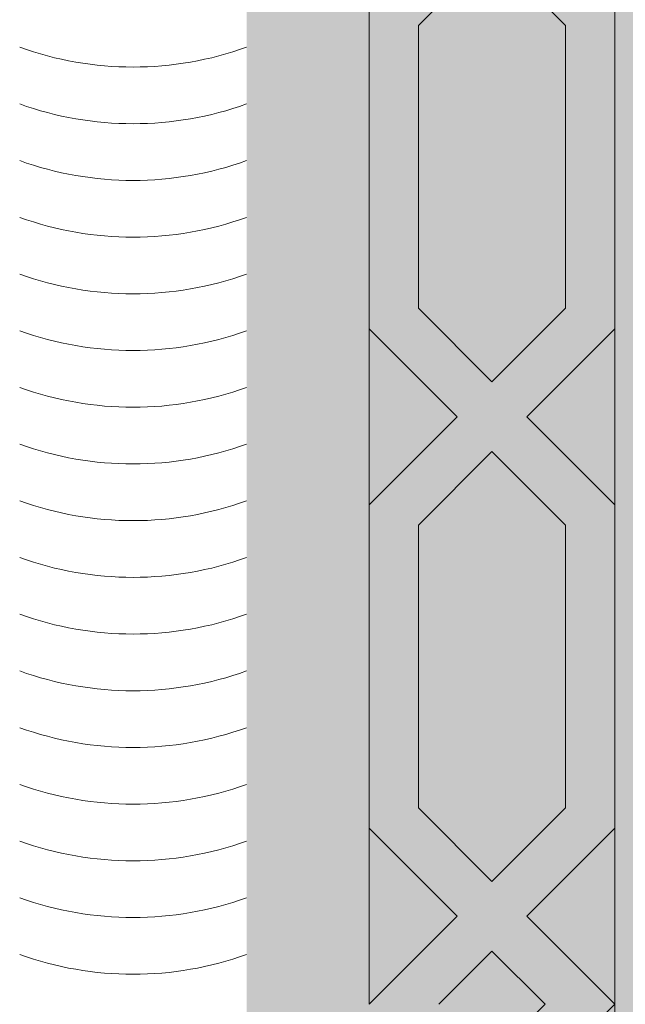
# Model space of a CAD drawing. Units: inches. Extents: x 844 to 2234, y 346 to 1084.
# Tile 56 of 93: x 1861.148 to 1864.294, y 701.365 to 706.48. Entities that reach past the tile are written whole.
import ezdxf

# ---------------------------------------------------------------- set-up
doc = ezdxf.new("R2010")
doc.units = ezdxf.units.IN
doc.header["$MEASUREMENT"] = 0
doc.layers.add('furniture', color=8, linetype='Continuous', lineweight=18)
doc.layers.add('RA-AP-01$0$INT', color=35, linetype='Continuous', lineweight=5)
doc.layers.add('RA-AP-01$0$FURN', color=3, linetype='Continuous')

# ---------------------------------------------------------------- blocks, each defined once
blk = doc.blocks.new('A$C18D01794')
at = {"layer": 'RA-AP-01$0$INT'}
h = blk.add_hatch(color=256, dxfattribs=at)
h.paths.add_polyline_path([(4.355206456958071, -6.156712009588037), (4.355206456958071, -8.056712009588038), (5.455206456958072, -8.056712009588038), (5.455206456958072, -6.156712009588037)])
h.paths.add_polyline_path([(4.405206456958072, -8.006712009588039), (4.405206456958072, -6.206712009588038), (5.405206456958072, -6.206712009588038), (5.405206456958072, -8.006712009588039)], flags=16)
h = blk.add_hatch(color=256, dxfattribs=at)
h.paths.add_polyline_path([(4.469348592586677, -7.07085414521094), (4.505206456958073, -7.03499628085108), (4.505206456958071, -7.106712009593861)])
h.paths.add_polyline_path([(4.455206456960671, -7.084996280832395), (4.476922185709333, -7.106712009588038), (4.433490728198045, -7.106712009588038)])
h.paths.add_polyline_path([(4.405206456958073, -7.034996280813718), (4.441064321339218, -7.070854145206393), (4.40520645695807, -7.106712009576003)])
h.paths.add_polyline_path([(4.425206456989053, -6.911460746921742), (4.455206456990736, -6.881460746929706), (4.485206456989055, -6.911460746937677), (4.48520645696979, -7.026712009590022), (4.455206456965227, -7.056712009584936), (4.425206456969784, -7.026712009579853)])
h.paths.add_polyline_path([(4.505206456958073, -6.831460746955388), (4.505206456958071, -6.903176475661116), (4.469348592616738, -6.867318611308251)])
h.paths.add_polyline_path([(4.425206456964688, -6.707925213036777), (4.455206456964794, -6.677925213027025), (4.485206456964689, -6.707925213017265), (4.485206456983951, -6.823176475683938), (4.455206456990736, -6.853176475686799), (4.425206456983956, -6.823176475689667)])
h.paths.add_polyline_path([(4.425206456974126, -6.504389679118949), (4.455206456959092, -6.474389679124341), (4.485206456974132, -6.504389679129721), (4.485206456993396, -6.619640941768059), (4.45520645699153, -6.649640941779566), (4.425206456993394, -6.619640941791077)])
h.paths.add_polyline_path([(4.46934859260189, -6.663783077416661), (4.505206456958071, -6.627925213048953), (4.505206456958073, -6.699640941761311)])
h.paths.add_polyline_path([(4.405206456958073, -6.627925213005104), (4.441064321354427, -6.663783077389926), (4.405206456958072, -6.699640941797813)])
h.paths.add_polyline_path([(4.405206456958072, -6.424389679139403), (4.441064321333084, -6.460247543502882), (4.405206456958072, -6.496105407889427)])
h.paths.add_polyline_path([(4.469348592580547, -6.460247543498336), (4.505206456958071, -6.424389679109282), (4.505206456958071, -6.496105407864332)])
h.paths.add_polyline_path([(4.425206456957888, -6.300854145208262), (4.45520645695415, -6.270854145221655), (4.485206456959507, -6.300854145217359), (4.48520645695824, -6.416105407863534), (4.455206456954537, -6.44610540787688), (4.425206456957888, -6.416105407889874)])
h.paths.add_polyline_path([(4.425206456957888, -6.226712009591025), (4.471064321332215, -6.226712009591025), (4.425206456957888, -6.272569873980103)])
h.paths.add_polyline_path([(4.499348592575121, -6.226712009591029), (4.636064321343707, -6.226712009591025), (4.666064321342317, -6.256712009589254), (4.636064321340932, -6.286712009591028), (4.499348592588945, -6.286712009591028), (4.469348592591685, -6.256712009584116)])
h.paths.add_polyline_path([(4.680206456964641, -6.270854145214393), (4.716064321337824, -6.306712009588038), (4.644348592591454, -6.306712009588038)])
h.paths.add_polyline_path([(4.644348592588108, -6.206712009588038), (4.716064321341167, -6.206712009588038), (4.680206456964637, -6.242569873964111)])
h.paths.add_polyline_path([(4.724348592586768, -6.226712009589824), (4.861064321340514, -6.226712009589824), (4.891064321340324, -6.256712009589255), (4.861064321340141, -6.286712009589827), (4.724348592587134, -6.286712009589821), (4.694348592586957, -6.256712009589254)])
h.paths.add_polyline_path([(4.905206456964143, -6.270854145212892), (4.941064321338827, -6.306712009588038), (4.869348592589457, -6.306712009588039)])
h.paths.add_polyline_path([(4.869348592586113, -6.206712009588038), (4.941064321342172, -6.206712009588038), (4.905206456964145, -6.242569873965612)])
h.paths.add_polyline_path([(4.949348592587774, -6.226712009589824), (5.086064321341521, -6.226712009589824), (5.116064321341329, -6.256712009589252), (5.08606432134115, -6.286712009589823), (4.949348592588145, -6.286712009589827), (4.919348592587961, -6.256712009589255)])
h.paths.add_polyline_path([(5.130206456963645, -6.270854145214393), (5.166064321336834, -6.306712009588038), (5.094348592590464, -6.306712009588038)])
h.paths.add_polyline_path([(5.094348592587119, -6.206712009588038), (5.166064321340178, -6.206712009588038), (5.130206456963651, -6.242569873964107)])
h.paths.add_polyline_path([(5.174348592584578, -6.226712009591027), (5.311064321353163, -6.226712009591027), (5.341064321336602, -6.256712009584116), (5.31106432133934, -6.286712009591028), (5.174348592587352, -6.286712009591028), (5.144348592585969, -6.256712009589254)])
h.paths.add_polyline_path([(5.325206456968778, -6.300854145217359), (5.355206456974136, -6.270854145221653), (5.385206456970396, -6.300854145208262), (5.385206456970396, -6.416105407889878), (5.355206456973747, -6.44610540787688), (5.325206456970044, -6.416105407863533)])
h.paths.add_polyline_path([(5.339348592596073, -6.226712009591029), (5.385206456970396, -6.226712009591025), (5.385206456970398, -6.272569873980105)])
h.paths.add_polyline_path([(5.325206456954155, -6.504389679129722), (5.355206456969194, -6.474389679124342), (5.38520645695416, -6.504389679118949), (5.385206456934896, -6.619640941791077), (5.355206456936758, -6.649640941779564), (5.325206456934888, -6.619640941768057)])
h.paths.add_polyline_path([(5.305206456958072, -6.424389679097139), (5.341064321347739, -6.460247543498338), (5.305206456958072, -6.496105407876472)])
h.paths.add_polyline_path([(5.369348592595204, -6.460247543502882), (5.40520645695807, -6.42438967915155), (5.405206456958072, -6.496105407877278)])
h.paths.add_polyline_path([(5.405206456958072, -6.627925213017245), (5.405206456958072, -6.69964094178567), (5.369348592573857, -6.663783077389926)])
h.paths.add_polyline_path([(5.305206456958072, -6.62792521303681), (5.341064321326393, -6.663783077416663), (5.305206456958072, -6.69964094177345)])
h.paths.add_polyline_path([(5.325206456963599, -6.707925213017267), (5.355206456963494, -6.677925213027021), (5.385206456963598, -6.707925213036775), (5.385206456944334, -6.823176475689665), (5.355206456937552, -6.853176475686797), (5.325206456944333, -6.823176475683936)])
h.paths.add_polyline_path([(5.305206456958072, -6.831460746943246), (5.341064321311551, -6.867318611308252), (5.305206456958072, -6.903176475673257)])
h.paths.add_polyline_path([(5.325206456939231, -6.911460746937672), (5.355206456937552, -6.881460746929707), (5.385206456939235, -6.911460746921742), (5.385206456958502, -7.026712009579853), (5.355206456963061, -7.056712009584934), (5.3252064569585, -7.026712009590026)])
h.paths.add_polyline_path([(5.404581768715993, -6.832085435167151, 0.001217816984214), (5.405206456958072, -6.832312009593747), (5.405206456958072, -6.90317647569123), (5.369348592563558, -6.867318611308251)])
h.paths.add_polyline_path([(5.36934859258907, -7.070854145206393), (5.40520645695807, -7.034996280825861), (5.405206456958072, -7.106712009563858)])
h.paths.add_polyline_path([(5.355206456967613, -7.084996280832394), (5.376922185730239, -7.106712009588038), (5.333490728218953, -7.106712009588036)])
h.paths.add_polyline_path([(5.30520645695807, -7.034996280838937), (5.341064321341609, -7.070854145210942), (5.305206456958074, -7.106712009606006)])
h = blk.add_hatch(color=256, dxfattribs=at)
h.paths.add_polyline_path([(4.505206456958071, -6.627925213048953), (4.46934859260189, -6.663783077416663), (4.505206456958071, -6.699640941761309), (4.505206456958071, -6.831460746955389), (4.469348592616735, -6.867318611308252), (4.505206456958071, -6.903176475661112), (4.505206456958071, -7.03499628085108), (4.469348592586679, -7.070854145210939), (4.505206456952245, -7.106712009588038), (4.476922185709333, -7.106712009588038), (4.455206456960671, -7.084996280832395), (4.433490728198047, -7.106712009588038), (4.405206456946033, -7.10671200958804), (4.441064321339216, -7.070854145206393), (4.40520645695807, -7.034996280813718), (4.405206456958072, -6.903176475703379), (4.441064321364728, -6.867318611308251), (4.40520645695807, -6.83146074691313), (4.40520645695807, -6.699640941797813), (4.441064321354429, -6.663783077389924), (4.405206456958072, -6.627925213005102), (4.405206456958072, -6.496105407889425), (4.441064321333084, -6.460247543502882), (4.405206456958072, -6.424389679139403), (4.405206456958072, -6.206712009588038), (4.644348592588106, -6.206712009588038), (4.680206456964639, -6.242569873964107), (4.716064321341165, -6.206712009588038), (4.869348592586113, -6.206712009588038), (4.905206456964143, -6.24256987396561), (4.941064321342174, -6.206712009588038), (5.094348592587118, -6.206712009588038), (5.130206456963649, -6.242569873964107), (5.166064321340178, -6.206712009588038), (5.405206456958072, -6.206712009588038), (5.405206456958072, -6.42438967915155), (5.369348592595202, -6.46024754350288), (5.40520645695807, -6.49610540787728), (5.40520645695807, -6.627925213017247), (5.369348592573859, -6.663783077389926), (5.40520645695807, -6.699640941785666), (5.40520645695807, -6.831460746925273), (5.36934859256356, -6.867318611308252), (5.405206456958072, -6.90317647569123), (5.405206456958072, -7.034996280825859), (5.369348592589068, -7.070854145206395), (5.405206456982249, -7.106712009588038), (5.376922185730244, -7.106712009588038), (5.355206456967613, -7.084996280832397), (5.333490728218955, -7.106712009588036), (5.305206456976043, -7.106712009588035), (5.341064321341609, -7.07085414521094), (5.305206456958072, -7.034996280838935), (5.305206456958072, -6.90317647567326), (5.34106432131155, -6.867318611308252), (5.305206456958072, -6.831460746943244), (5.30520645695807, -6.699640941773452), (5.341064321326395, -6.663783077416663), (5.305206456958072, -6.627925213036814), (5.305206456958072, -6.496105407876472), (5.341064321347738, -6.46024754349834), (5.305206456958072, -6.424389679097137), (5.30520645695807, -6.306712009588038), (5.166064321336834, -6.306712009588038), (5.130206456963647, -6.270854145214393), (5.094348592590464, -6.306712009588038), (4.941064321338827, -6.306712009588036), (4.905206456964145, -6.270854145212892), (4.869348592589459, -6.306712009588038), (4.716064321337822, -6.306712009588036), (4.680206456964641, -6.270854145214393), (4.644348592591453, -6.306712009588038), (4.505206456958071, -6.306712009588038), (4.505206456958071, -6.424389679109282), (4.469348592580545, -6.460247543498338), (4.505206456958071, -6.496105407864328)])
h.paths.add_polyline_path([(4.485206456974132, -6.504389679129722), (4.45520645695909, -6.474389679124341), (4.425206456974128, -6.504389679118945), (4.425206456993394, -6.619640941791079), (4.45520645699153, -6.649640941779566), (4.485206456993396, -6.619640941768059)], flags=16)
h.paths.add_polyline_path([(4.455206456954537, -6.44610540787688), (4.485206456958242, -6.416105407863534), (4.48520645695951, -6.30085414521736), (4.45520645695415, -6.270854145221653), (4.425206456957888, -6.300854145208264), (4.425206456957888, -6.41610540788988)], flags=16)
h.paths.add_polyline_path([(4.455206456964794, -6.677925213027025), (4.42520645696469, -6.707925213036777), (4.425206456983954, -6.82317647568967), (4.455206456990734, -6.853176475686797), (4.485206456983953, -6.823176475683936), (4.485206456964687, -6.707925213017265)], flags=16)
h.paths.add_polyline_path([(4.499348592588947, -6.286712009591028), (4.636064321340932, -6.286712009591028), (4.666064321342317, -6.256712009589254), (4.636064321343707, -6.226712009591027), (4.499348592575121, -6.226712009591029), (4.469348592591685, -6.256712009584118)], flags=16)
h.paths.add_polyline_path([(4.425206456957888, -6.272569873980103), (4.471064321332215, -6.226712009591025), (4.425206456957888, -6.226712009591025)], flags=16)
h.paths.add_polyline_path([(4.455206456990734, -6.881460746929709), (4.425206456989053, -6.91146074692174), (4.425206456969784, -7.026712009579853), (4.455206456965226, -7.056712009584932), (4.485206456969787, -7.026712009590026), (4.485206456989053, -6.911460746937672)], flags=16)
h.paths.add_polyline_path([(4.72434859258714, -6.286712009589821), (4.861064321340141, -6.286712009589829), (4.891064321340324, -6.256712009589254), (4.861064321340513, -6.226712009589823), (4.724348592586768, -6.226712009589823), (4.694348592586956, -6.256712009589254)], flags=16)
h.paths.add_polyline_path([(4.919348592587961, -6.256712009589254), (4.949348592588145, -6.286712009589827), (5.08606432134115, -6.286712009589823), (5.116064321341327, -6.256712009589254), (5.086064321341519, -6.226712009589824), (4.949348592587774, -6.226712009589824)], flags=16)
h.paths.add_polyline_path([(5.144348592585967, -6.256712009589254), (5.174348592587358, -6.286712009591028), (5.311064321339338, -6.286712009591028), (5.3410643213366, -6.256712009584118), (5.311064321353163, -6.226712009591029), (5.174348592584576, -6.226712009591027)], flags=16)
h.paths.add_polyline_path([(5.32520645693489, -6.619640941768055), (5.355206456936755, -6.649640941779566), (5.385206456934894, -6.619640941791079), (5.38520645695416, -6.504389679118949), (5.355206456969194, -6.474389679124341), (5.325206456954153, -6.504389679129724)], flags=16)
h.paths.add_polyline_path([(5.325206456970042, -6.416105407863534), (5.355206456973747, -6.44610540787688), (5.385206456970398, -6.416105407889876), (5.385206456970398, -6.30085414520826), (5.355206456974136, -6.270854145221653), (5.325206456968778, -6.30085414521736)], flags=16)
h.paths.add_polyline_path([(5.325206456963599, -6.707925213017265), (5.325206456944333, -6.823176475683936), (5.355206456937552, -6.853176475686797), (5.385206456944332, -6.823176475689667), (5.385206456963596, -6.707925213036773), (5.355206456963492, -6.677925213027027)], flags=16)
h.paths.add_polyline_path([(5.32520645693923, -6.911460746937674), (5.3252064569585, -7.026712009590026), (5.355206456963062, -7.056712009584934), (5.3852064569585, -7.026712009579853), (5.385206456939234, -6.911460746921738), (5.355206456937552, -6.881460746929707)], flags=16)
h.paths.add_polyline_path([(5.339348592596071, -6.226712009591029), (5.385206456970398, -6.272569873980103), (5.385206456970396, -6.226712009591027)], flags=16)
for points in [[(4.505206456958071, -6.306712009588038), (5.305206456958072, -6.306712009588038), (5.305206456958072, -7.106712009588038), (5.255206456951893, -7.10671200958804), (5.25520645694868, -6.356712009605972), (4.555206456959269, -6.356712009587461), (4.555206456956052, -7.106712009588038), (4.505206456958073, -7.106712009588038)], [(4.505206456958071, -7.906712009588039), (5.305206456958072, -7.906712009588039), (5.305206456958072, -7.106712009588038), (5.255206456951893, -7.106712009588036), (5.25520645694868, -7.856712009570104), (4.555206456959269, -7.856712009588616), (4.555206456956052, -7.106712009588038), (4.505206456958073, -7.106712009588038)], [(4.405206456958072, -7.381963272262946), (4.441064321364729, -7.346105407867824), (4.405206456958072, -7.310247543472702)]]:
    blk.add_hatch(color=256, dxfattribs=at).paths.add_polyline_path(points)
h = blk.add_hatch(color=256, dxfattribs=at)
h.paths.add_polyline_path([(4.505206456958071, -7.585498806127123), (4.46934859260189, -7.549640941759413), (4.505206456958071, -7.513783077414768), (4.505206456958071, -7.381963272220687), (4.469348592616735, -7.346105407867824), (4.505206456958071, -7.310247543514964), (4.505206456958071, -7.178427738324996), (4.469348592586679, -7.142569873965138), (4.505206456952245, -7.106712009588038), (4.476922185709333, -7.106712009588038), (4.455206456960671, -7.128427738343681), (4.433490728198047, -7.106712009588038), (4.405206456946033, -7.106712009588036), (4.441064321339216, -7.142569873969684), (4.40520645695807, -7.178427738362358), (4.405206456958072, -7.310247543472698), (4.441064321364728, -7.346105407867826), (4.40520645695807, -7.381963272262947), (4.40520645695807, -7.513783077378263), (4.441064321354429, -7.549640941786153), (4.405206456958072, -7.585498806170974), (4.405206456958072, -7.717318611286652), (4.441064321333084, -7.753176475673194), (4.405206456958072, -7.789034340036673), (4.405206456958072, -8.006712009588039), (4.644348592588106, -8.006712009588039), (4.680206456964639, -7.970854145211967), (4.716064321341165, -8.006712009588039), (4.869348592586113, -8.006712009588039), (4.905206456964143, -7.970854145210465), (4.941064321342174, -8.006712009588039), (5.094348592587118, -8.006712009588037), (5.130206456963649, -7.970854145211967), (5.166064321340178, -8.006712009588039), (5.405206456958072, -8.006712009588039), (5.405206456958072, -7.789034340024526), (5.369348592595202, -7.753176475673196), (5.40520645695807, -7.717318611298797), (5.40520645695807, -7.585498806158829), (5.369348592573859, -7.549640941786151), (5.40520645695807, -7.51378307739041), (5.40520645695807, -7.381963272250803), (5.36934859256356, -7.346105407867824), (5.405206456958072, -7.310247543484846), (5.405206456958072, -7.178427738350217), (5.369348592589068, -7.142569873969682), (5.405206456982249, -7.106712009588038), (5.376922185730244, -7.106712009588038), (5.355206456967613, -7.128427738343679), (5.333490728218955, -7.10671200958804), (5.305206456976043, -7.106712009588042), (5.341064321341609, -7.142569873965136), (5.305206456958072, -7.178427738337141), (5.305206456958072, -7.310247543502816), (5.34106432131155, -7.346105407867824), (5.305206456958072, -7.381963272232832), (5.30520645695807, -7.513783077402624), (5.341064321326395, -7.549640941759413), (5.305206456958072, -7.585498806139263), (5.305206456958072, -7.717318611299605), (5.341064321347738, -7.753176475677737), (5.305206456958072, -7.78903434007894), (5.30520645695807, -7.906712009588039), (5.166064321336834, -7.906712009588039), (5.130206456963647, -7.942569873961684), (5.094348592590464, -7.906712009588039), (4.941064321338827, -7.906712009588041), (4.905206456964145, -7.942569873963183), (4.869348592589459, -7.906712009588039), (4.716064321337822, -7.906712009588041), (4.680206456964641, -7.942569873961684), (4.644348592591453, -7.906712009588039), (4.505206456958071, -7.906712009588039), (4.505206456958071, -7.789034340066795), (4.469348592580545, -7.753176475677738), (4.505206456958071, -7.717318611311748)])
h.paths.add_polyline_path([(4.485206456974132, -7.709034340046354), (4.45520645695909, -7.739034340051736), (4.425206456974128, -7.709034340057131), (4.425206456993394, -7.593783077384998), (4.45520645699153, -7.563783077396511), (4.485206456993396, -7.593783077408017)], flags=16)
h.paths.add_polyline_path([(4.455206456954537, -7.767318611299197), (4.485206456958242, -7.797318611312542), (4.48520645695951, -7.912569873958716), (4.45520645695415, -7.942569873954422), (4.425206456957888, -7.912569873967813), (4.425206456957888, -7.797318611286197)], flags=16)
h.paths.add_polyline_path([(4.455206456964794, -7.535498806149051), (4.42520645696469, -7.5054988061393), (4.425206456983954, -7.390247543486406), (4.455206456990734, -7.360247543489279), (4.485206456983953, -7.39024754349214), (4.485206456964687, -7.505498806158811)], flags=16)
h.paths.add_polyline_path([(4.499348592588947, -7.926712009585049), (4.636064321340932, -7.926712009585049), (4.666064321342317, -7.956712009586821), (4.636064321343707, -7.986712009585048), (4.499348592575121, -7.986712009585048), (4.469348592591685, -7.956712009591957)], flags=16)
h.paths.add_polyline_path([(4.425206456957888, -7.940854145195974), (4.471064321332215, -7.986712009585049), (4.425206456957888, -7.986712009585049)], flags=16)
h.paths.add_polyline_path([(4.455206456990734, -7.331963272246367), (4.425206456989053, -7.301963272254337), (4.425206456969784, -7.186712009596224), (4.455206456965226, -7.156712009591144), (4.485206456969787, -7.186712009586051), (4.485206456989053, -7.301963272238404)], flags=16)
h.paths.add_polyline_path([(4.72434859258714, -7.926712009586255), (4.861064321340141, -7.926712009586248), (4.891064321340324, -7.956712009586823), (4.861064321340513, -7.986712009586252), (4.724348592586768, -7.986712009586252), (4.694348592586956, -7.956712009586821)], flags=16)
h.paths.add_polyline_path([(4.919348592587961, -7.956712009586821), (4.949348592588145, -7.92671200958625), (5.08606432134115, -7.926712009586253), (5.116064321341327, -7.956712009586823), (5.086064321341519, -7.986712009586252), (4.949348592587774, -7.986712009586252)], flags=16)
h.paths.add_polyline_path([(5.144348592585967, -7.956712009586823), (5.174348592587358, -7.926712009585049), (5.311064321339338, -7.926712009585049), (5.3410643213366, -7.956712009591957), (5.311064321353163, -7.986712009585048), (5.174348592584576, -7.986712009585048)], flags=16)
h.paths.add_polyline_path([(5.32520645693489, -7.593783077408021), (5.355206456936755, -7.563783077396511), (5.385206456934894, -7.593783077384998), (5.38520645695416, -7.709034340057128), (5.355206456969194, -7.739034340051736), (5.325206456954153, -7.709034340046352)], flags=16)
h.paths.add_polyline_path([(5.325206456970042, -7.797318611312542), (5.355206456973747, -7.767318611299197), (5.385206456970398, -7.7973186112862), (5.385206456970398, -7.912569873967816), (5.355206456974136, -7.942569873954422), (5.325206456968778, -7.912569873958716)], flags=16)
h.paths.add_polyline_path([(5.325206456963599, -7.505498806158811), (5.325206456944333, -7.39024754349214), (5.355206456937552, -7.360247543489279), (5.385206456944332, -7.39024754348641), (5.385206456963596, -7.505498806139303), (5.355206456963492, -7.53549880614905)], flags=16)
h.paths.add_polyline_path([(5.32520645693923, -7.301963272238403), (5.3252064569585, -7.186712009586051), (5.355206456963062, -7.156712009591142), (5.3852064569585, -7.186712009596224), (5.385206456939234, -7.301963272254338), (5.355206456937552, -7.331963272246369)], flags=16)
h.paths.add_polyline_path([(5.339348592596071, -7.986712009585048), (5.385206456970398, -7.940854145195972), (5.385206456970396, -7.986712009585048)], flags=16)
h = blk.add_hatch(color=256, dxfattribs=at)
h.paths.add_polyline_path([(4.469348592586677, -7.142569873965136), (4.505206456958073, -7.178427738324996), (4.505206456958071, -7.106712009582215)])
h.paths.add_polyline_path([(4.455206456960671, -7.128427738343681), (4.476922185709333, -7.106712009588038), (4.433490728198045, -7.106712009588038)])
h.paths.add_polyline_path([(4.405206456958073, -7.178427738362358), (4.441064321339218, -7.142569873969684), (4.40520645695807, -7.106712009600073)])
h.paths.add_polyline_path([(4.425206456989053, -7.301963272254335), (4.455206456990736, -7.331963272246371), (4.485206456989055, -7.301963272238399), (4.48520645696979, -7.186712009586054), (4.455206456965227, -7.15671200959114), (4.425206456969784, -7.186712009596224)])
h.paths.add_polyline_path([(4.505206456958073, -7.381963272220689), (4.505206456958071, -7.310247543514961), (4.469348592616738, -7.346105407867826)])
h.paths.add_polyline_path([(4.425206456964688, -7.5054988061393), (4.455206456964794, -7.535498806149051), (4.485206456964689, -7.505498806158811), (4.485206456983951, -7.390247543492138), (4.455206456990736, -7.360247543489277), (4.425206456983956, -7.39024754348641)])
h.paths.add_polyline_path([(4.425206456974126, -7.709034340057128), (4.455206456959092, -7.739034340051736), (4.485206456974132, -7.709034340046356), (4.485206456993396, -7.593783077408017), (4.45520645699153, -7.563783077396511), (4.425206456993394, -7.593783077384999)])
h.paths.add_polyline_path([(4.46934859260189, -7.549640941759415), (4.505206456958071, -7.585498806127123), (4.505206456958073, -7.513783077414766)])
h.paths.add_polyline_path([(4.405206456958073, -7.585498806170972), (4.441064321354427, -7.549640941786151), (4.405206456958072, -7.513783077378263)])
h.paths.add_polyline_path([(4.405206456958072, -7.789034340036673), (4.441064321333084, -7.753176475673194), (4.405206456958072, -7.71731861128665)])
h.paths.add_polyline_path([(4.469348592580547, -7.75317647567774), (4.505206456958071, -7.789034340066795), (4.505206456958071, -7.717318611311744)])
h.paths.add_polyline_path([(4.425206456957888, -7.912569873967814), (4.45520645695415, -7.942569873954422), (4.485206456959507, -7.912569873958718), (4.48520645695824, -7.797318611312542), (4.455206456954537, -7.767318611299197), (4.425206456957888, -7.797318611286202)])
h.paths.add_polyline_path([(4.425206456957888, -7.986712009585049), (4.471064321332215, -7.986712009585049), (4.425206456957888, -7.940854145195972)])
h.paths.add_polyline_path([(4.499348592575121, -7.986712009585048), (4.636064321343707, -7.986712009585049), (4.666064321342317, -7.956712009586823), (4.636064321340932, -7.926712009585049), (4.499348592588945, -7.926712009585049), (4.469348592591685, -7.95671200959196)])
h.paths.add_polyline_path([(4.680206456964641, -7.942569873961684), (4.716064321337824, -7.906712009588039), (4.644348592591454, -7.906712009588039)])
h.paths.add_polyline_path([(4.644348592588108, -8.006712009588039), (4.716064321341167, -8.006712009588039), (4.680206456964637, -7.970854145211964)])
h.paths.add_polyline_path([(4.724348592586768, -7.98671200958625), (4.861064321340514, -7.986712009586252), (4.891064321340324, -7.956712009586819), (4.861064321340141, -7.92671200958625), (4.724348592587134, -7.926712009586255), (4.694348592586957, -7.956712009586821)])
h.paths.add_polyline_path([(4.905206456964143, -7.942569873963183), (4.941064321338827, -7.906712009588039), (4.869348592589457, -7.906712009588037)])
h.paths.add_polyline_path([(4.869348592586113, -8.006712009588039), (4.941064321342172, -8.006712009588037), (4.905206456964145, -7.970854145210463)])
h.paths.add_polyline_path([(4.949348592587774, -7.986712009586252), (5.086064321341521, -7.986712009586252), (5.116064321341329, -7.956712009586823), (5.08606432134115, -7.926712009586253), (4.949348592588145, -7.92671200958625), (4.919348592587961, -7.956712009586819)])
h.paths.add_polyline_path([(5.130206456963645, -7.942569873961684), (5.166064321336834, -7.906712009588039), (5.094348592590464, -7.906712009588039)])
h.paths.add_polyline_path([(5.094348592587119, -8.006712009588039), (5.166064321340178, -8.006712009588039), (5.130206456963651, -7.970854145211967)])
h.paths.add_polyline_path([(5.174348592584578, -7.986712009585048), (5.311064321353163, -7.986712009585048), (5.341064321336602, -7.956712009591958), (5.31106432133934, -7.926712009585049), (5.174348592587352, -7.926712009585049), (5.144348592585969, -7.956712009586823)])
h.paths.add_polyline_path([(5.325206456968778, -7.912569873958718), (5.355206456974136, -7.942569873954422), (5.385206456970396, -7.912569873967814), (5.385206456970396, -7.797318611286199), (5.355206456973747, -7.767318611299197), (5.325206456970044, -7.797318611312544)])
h.paths.add_polyline_path([(5.339348592596073, -7.986712009585048), (5.385206456970396, -7.986712009585049), (5.385206456970398, -7.94085414519597)])
h.paths.add_polyline_path([(5.325206456954155, -7.709034340046354), (5.355206456969194, -7.739034340051734), (5.38520645695416, -7.709034340057128), (5.385206456934896, -7.593783077384999), (5.355206456936758, -7.563783077396513), (5.325206456934888, -7.593783077408019)])
h.paths.add_polyline_path([(5.305206456958072, -7.789034340078938), (5.341064321347739, -7.753176475677738), (5.305206456958072, -7.717318611299605)])
h.paths.add_polyline_path([(5.369348592595204, -7.753176475673194), (5.40520645695807, -7.789034340024526), (5.405206456958072, -7.717318611298798)])
h.paths.add_polyline_path([(5.405206456958072, -7.585498806158831), (5.405206456958072, -7.513783077390407), (5.369348592573857, -7.549640941786151)])
h.paths.add_polyline_path([(5.305206456958072, -7.585498806139266), (5.341064321326393, -7.549640941759413), (5.305206456958072, -7.513783077402626)])
h.paths.add_polyline_path([(5.325206456963599, -7.50549880615881), (5.355206456963494, -7.535498806149055), (5.385206456963598, -7.505498806139302), (5.385206456944334, -7.390247543486411), (5.355206456937552, -7.360247543489279), (5.325206456944333, -7.39024754349214)])
h.paths.add_polyline_path([(5.305206456958072, -7.38196327223283), (5.341064321311551, -7.346105407867824), (5.305206456958072, -7.31024754350282)])
h.paths.add_polyline_path([(5.325206456939231, -7.301963272238404), (5.355206456937552, -7.331963272246369), (5.385206456939235, -7.301963272254335), (5.385206456958502, -7.186712009596224), (5.355206456963061, -7.156712009591142), (5.3252064569585, -7.186712009586051)])
h.paths.add_polyline_path([(5.404581768715993, -7.381338584008926, -0.001217816984214), (5.405206456958072, -7.381112009582329), (5.405206456958072, -7.310247543484846), (5.369348592563558, -7.346105407867826)])
h.paths.add_polyline_path([(5.36934859258907, -7.142569873969684), (5.40520645695807, -7.178427738350215), (5.405206456958072, -7.106712009612218)])
h.paths.add_polyline_path([(5.355206456967613, -7.128427738343683), (5.376922185730239, -7.106712009588038), (5.333490728218953, -7.10671200958804)])
h.paths.add_polyline_path([(5.30520645695807, -7.178427738337139), (5.341064321341609, -7.142569873965134), (5.305206456958074, -7.10671200957007)])
for p, q in [((4.469348592586677, -7.07085414521094), (4.505206456958071, -7.106712009593865)), ((4.455206456960673, -7.084996280832395), (4.476922185709333, -7.106712009588038)), ((4.441064321339218, -7.142569873969684), (4.405206456956286, -7.10671200959829)), ((4.455206456960673, -7.128427738343681), (4.433490728204252, -7.106712009594245)), ((4.455206456960673, -7.128427738343681), (4.476922185709333, -7.106712009588038)), ((4.469348592586677, -7.142569873965136), (4.505206456958071, -7.106712009582212)), ((4.405206456969147, -7.178427738351285), (4.441064321339218, -7.142569873969684)), ((4.505206456969147, -7.178427738336072), (4.469348592586681, -7.14256987396514)), ((4.425206456970426, -7.186712009595584), (4.455206456965226, -7.156712009591142)), ((4.485206456970428, -7.186712009586692), (4.455206456965226, -7.156712009591142)), ((4.425206456989053, -7.301963272254337), (4.425206456969786, -7.186712009596725)), ((4.485206456989055, -7.301963272238403), (4.485206456969787, -7.186712009586692)), ((4.425206456989053, -7.301963272254337), (4.455206456990734, -7.331963272246369)), ((4.485206456989055, -7.301963272238403), (4.455206456990734, -7.331963272246369)), ((4.405206456987673, -7.310247543502303), (4.441064321369275, -7.346105407872371)), ((4.505206456987672, -7.31024754348536), (4.469348592616737, -7.346105407867824)), ((4.405206456987673, -7.381963272233345), (4.441064321369275, -7.346105407863277)), ((4.505206456987672, -7.381963272250288), (4.469348592616737, -7.346105407867824)), ((4.425206456983954, -7.39024754348641), (4.455206456990734, -7.360247543489279)), ((4.485206456983953, -7.39024754349214), (4.455206456990734, -7.360247543489279)), ((4.425206456983954, -7.39024754348641), (4.425206456964688, -7.5054988061393)), ((4.485206456983953, -7.39024754349214), (4.485206456964687, -7.505498806158811)), ((4.425206456964688, -7.5054988061393), (4.455206456964796, -7.535498806149051)), ((4.485206456964687, -7.505498806158811), (4.455206456964796, -7.535498806149051))]:
    blk.add_line(p, q, dxfattribs=at)
for points in [[(5.305206456958072, -7.106712009588038), (5.305206456958072, -6.306712009588038), (4.505206456958071, -6.306712009588038), (4.505206456958071, -7.106712009588038)], [(5.405206456958072, -8.006712009588039), (4.405206456958072, -8.006712009588039), (4.405206456958072, -7.106712009588038)], [(5.305206456958072, -7.106712009588038), (5.305206456958072, -7.906712009588039), (4.505206456958071, -7.906712009588039), (4.505206456958071, -7.106712009588038)]]:
    blk.add_lwpolyline(points, dxfattribs=at)
for centre in [(4.309006456955269, -7.255364458282008), (4.309006456955269, -7.278464458280756), (4.309006456953677, -7.301564458285417), (4.309006456954814, -7.324664458284166), (4.309006456954814, -7.347764458279732), (4.309006456953222, -7.37086445828462), (4.309006456955951, -7.393964458283369), (4.309006456955951, -7.417064458282117), (4.309006456954359, -7.440164458286778), (4.309006456955496, -7.463264458285527), (4.309006456955496, -7.486364458281093), (4.309006456953905, -7.509464458285981), (4.309006456952086, -7.532564458284502), (4.309006456955041, -7.555664458280295), (4.309006456954814, -7.578764458284956), (4.309006456953222, -7.601864458283705), (4.309006456951631, -7.624964458285409)]:
    blk.add_arc(centre, 0.136414042854523, 70.20384312815696, 109.7961568705686, dxfattribs=at)
blk = doc.blocks.new('A$C5D2F253E')
at = {"layer": 'RA-AP-01$0$FURN', "xscale": -0.7999999999883585, "yscale": 0.7999999999883585, "zscale": 0.8, "rotation": 90}
blk.add_blockref('A$C18D01794', (-5.687757199772477, 4.75791982714071), dxfattribs=at)

msp = doc.modelspace()

# ---------------------------------------------------------------- block references
at = {"layer": 'furniture', "xscale": 15.94108302203742, "yscale": 15.94108302203742, "zscale": 15.94108302203742, "rotation": 90}
msp.add_blockref('A$C5D2F253E', (1882.631064852549, 701.4028671565849), dxfattribs=at)

doc.saveas('drawing.dxf')
